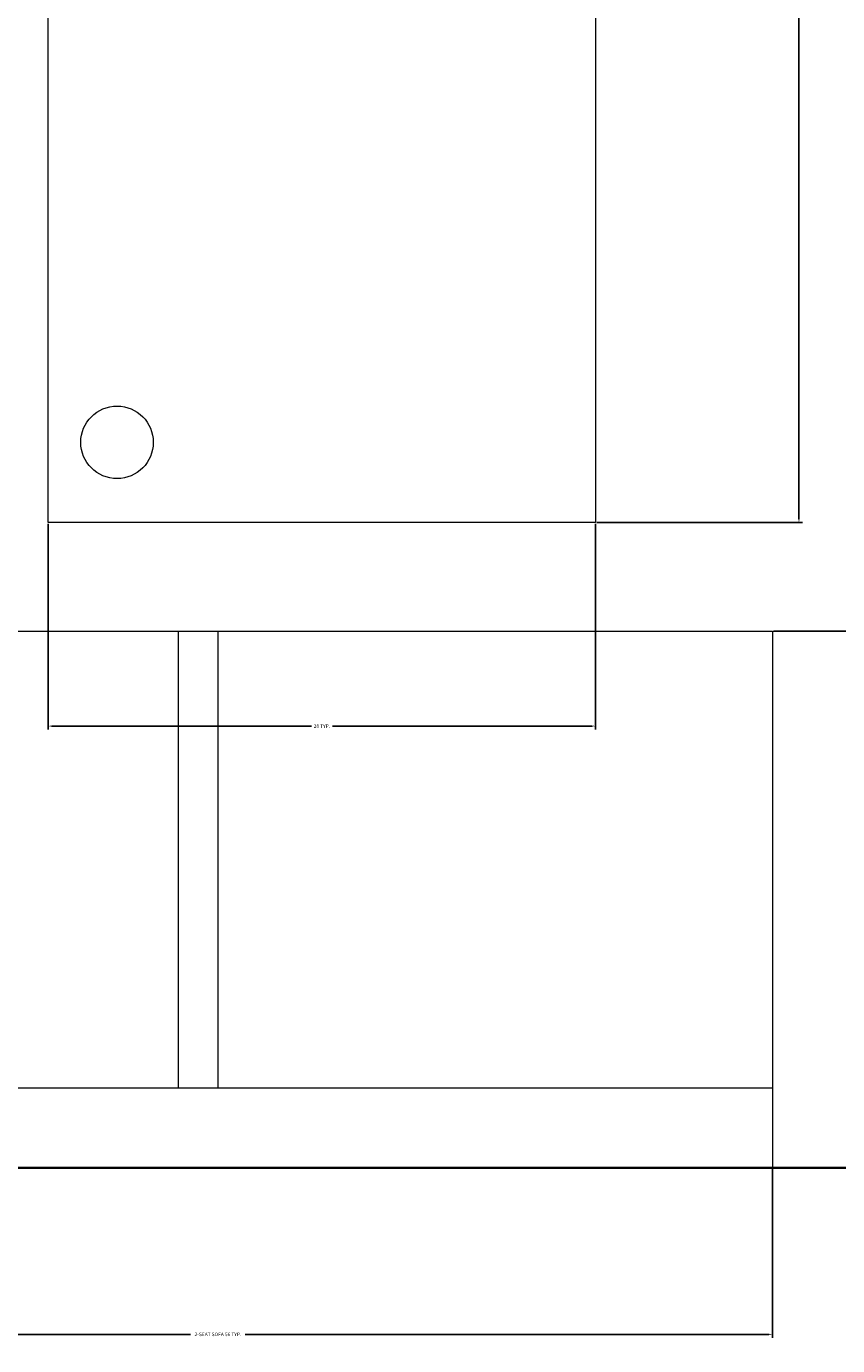
# Model space of a CAD drawing. Units: inches. Extents: x 108 to 613, y 1573 to 2319.
# Tile 5 of 11: x 365 to 406, y 1989 to 2055. Entities that reach past the tile are written whole.
import ezdxf

# ---------------------------------------------------------------- set-up
doc = ezdxf.new("R2010")
doc.units = ezdxf.units.IN
for name, color, linetype, lineweight in [('A-ANNO-DIMS', 2, 'Continuous', 18), ('furniture', 2, 'Continuous', 18), ('wall', 6, 'Continuous', 35)]:
    doc.layers.add(name, color=color, linetype=linetype, lineweight=lineweight)
doc.styles.get("Standard").update_dxf_attribs({"font": 'arial.ttf'})
doc.dimstyles.get("Standard").update_dxf_attribs({"dimtxt": 0.18, "dimasz": 0.18, "dimexe": 0.18, "dimexo": 0.0625, "dimgap": 0.09, "dimtad": 0, "dimtih": 1, "dimtoh": 1, "dimdec": 4, "dimzin": 0, "dimdsep": 46, "dimtxsty": 'Standard', "dimcen": 0.09, "dimadec": 0, "dimazin": 0, "dimtfac": 1, "dimtdec": 4, "dimtofl": 0, "dimtmove": 0, "dimatfit": 3, "dimfxl": 1, "dimtolj": 1, "dimtzin": 0, "dimarcsym": 0})

# ---------------------------------------------------------------- blocks, each defined once
blk = doc.blocks.new('COFFEE-TABLE')
blk.add_lwpolyline([(0, 68.458), (27.63, 68.458), (27.63, 0), (0, 0)], close=True)
blk.add_circle((3.474, 4.049), 1.83)
blk = doc.blocks.new('SOFA-2-SEAT')
for p, q in [((25.991, 27.084), (25.991, 4.025)), ((27.991, 27.084), (27.991, 4.025)), ((55.982, 4.025), (0, 4.025))]:
    blk.add_line(p, q)
blk.add_lwpolyline([(0, 27.084), (55.982, 27.084), (55.982, 0), (0, 0)], close=True)
blk = doc.blocks.new('*D29')
at = {"layer": 'A-ANNO-DIMS', "color": 0, "lineweight": -2, "transparency": 16777216}
for p, q in [((394.077, 2098.634), (404.464, 2098.634)), ((404.284, 2098.454), (404.284, 2064.588)), ((404.284, 2030.356), (404.284, 2064.222)), ((394.077, 2030.176), (404.464, 2030.176))]:
    blk.add_line(p, q, dxfattribs=at)
at = {"layer": 'A-ANNO-DIMS', "color": 0, "transparency": 16777216}
for points in [[(404.254, 2098.454), (404.314, 2098.454), (404.284, 2098.634)], [(404.254, 2030.356), (404.314, 2030.356), (404.284, 2030.176)]]:
    blk.add_solid(points, dxfattribs=at)
at = {"layer": 'Defpoints', "color": 0, "transparency": 16777216}
for p in [(394.015, 2098.634), (404.284, 2098.634), (394.015, 2030.176)]:
    blk.add_point(p, dxfattribs=at)
at = {"layer": 'A-ANNO-DIMS', "color": 0, "transparency": 16777216, "insert": (404.284, 2064.405), "char_height": 0.18, "attachment_point": 5}
blk.add_mtext('\\A1;COFFEE TABLE 68 TYP.', dxfattribs=at)
blk = doc.blocks.new('*D30')
at = {"layer": 'A-ANNO-DIMS', "color": 0, "lineweight": -2, "transparency": 16777216}
for p, q in [((366.385, 2030.114), (366.385, 2019.727)), ((394.015, 2030.114), (394.015, 2019.727)), ((366.565, 2019.907), (379.671, 2019.907)), ((393.835, 2019.907), (380.73, 2019.907))]:
    blk.add_line(p, q, dxfattribs=at)
at = {"layer": 'A-ANNO-DIMS', "color": 0, "transparency": 16777216}
for points in [[(366.565, 2019.937), (366.565, 2019.877), (366.385, 2019.907)], [(393.835, 2019.937), (393.835, 2019.877), (394.015, 2019.907)]]:
    blk.add_solid(points, dxfattribs=at)
at = {"layer": 'Defpoints', "color": 0, "transparency": 16777216}
for p in [(366.385, 2030.176), (394.015, 2030.176), (394.015, 2019.907)]:
    blk.add_point(p, dxfattribs=at)
at = {"layer": 'A-ANNO-DIMS', "color": 0, "transparency": 16777216, "insert": (380.2, 2019.907), "char_height": 0.18, "attachment_point": 5}
blk.add_mtext('\\A1;28 TYP.', dxfattribs=at)
blk = doc.blocks.new('*D33')
at = {"layer": 'A-ANNO-DIMS', "color": 0, "lineweight": -2, "transparency": 16777216}
for p, q in [((346.962, 1997.55), (346.962, 1989.035)), ((402.944, 1997.55), (402.944, 1989.035)), ((347.142, 1989.215), (373.571, 1989.215)), ((402.764, 1989.215), (376.335, 1989.215))]:
    blk.add_line(p, q, dxfattribs=at)
at = {"layer": 'A-ANNO-DIMS', "color": 0, "transparency": 16777216}
for points in [[(347.142, 1989.245), (347.142, 1989.185), (346.962, 1989.215)], [(402.764, 1989.245), (402.764, 1989.185), (402.944, 1989.215)]]:
    blk.add_solid(points, dxfattribs=at)
at = {"layer": 'Defpoints', "color": 0, "transparency": 16777216}
for p in [(346.962, 1997.612), (402.944, 1997.612), (402.944, 1989.215)]:
    blk.add_point(p, dxfattribs=at)
at = {"layer": 'A-ANNO-DIMS', "color": 0, "transparency": 16777216, "insert": (374.953, 1989.215), "char_height": 0.18, "attachment_point": 5}
blk.add_mtext('\\A1;2-SEAT SOFA 56 TYP.', dxfattribs=at)
blk = doc.blocks.new('*D34')
at = {"layer": 'A-ANNO-DIMS', "color": 0, "lineweight": -2, "transparency": 16777216}
for p, q in [((403.006, 2024.696), (411.521, 2024.696)), ((411.341, 2024.516), (411.341, 2011.335)), ((411.341, 1997.792), (411.341, 2010.974)), ((403.006, 1997.612), (411.521, 1997.612))]:
    blk.add_line(p, q, dxfattribs=at)
at = {"layer": 'A-ANNO-DIMS', "color": 0, "transparency": 16777216}
for points in [[(411.311, 2024.516), (411.371, 2024.516), (411.341, 2024.696)], [(411.311, 1997.792), (411.371, 1997.792), (411.341, 1997.612)]]:
    blk.add_solid(points, dxfattribs=at)
at = {"layer": 'Defpoints', "color": 0, "transparency": 16777216}
for p in [(402.944, 2024.696), (411.341, 2024.696), (402.944, 1997.612)]:
    blk.add_point(p, dxfattribs=at)
at = {"layer": 'A-ANNO-DIMS', "color": 0, "transparency": 16777216, "insert": (411.341, 2011.154), "char_height": 0.18, "attachment_point": 5}
blk.add_mtext('\\A1;27 TYP.', dxfattribs=at)

msp = doc.modelspace()

# ---------------------------------------------------------------- linework, layer by layer
at = {"layer": 'wall'}
msp.add_line((341.2753, 1997.6125), (431.2753, 1997.6125), dxfattribs=at)

# ---------------------------------------------------------------- block references
at = {"layer": 'furniture'}
for name, p in [('COFFEE-TABLE', (366.385, 2030.176)), ('SOFA-2-SEAT', (346.962, 1997.612))]:
    msp.add_blockref(name, p, dxfattribs=at)

# ---------------------------------------------------------------- dimensions: what is measured, and where the dimension line sits
at = {"layer": 'A-ANNO-DIMS'}
for base, p1, p2, text, picture, middle in [((404.2835, 2098.634), (394.0149, 2030.176), (394.0149, 2098.634), 'COFFEE TABLE <> TYP.', '*D29', (404.2835, 2064.405)), ((411.3411, 2024.6958), (402.9438, 1997.6125), (402.9438, 2024.6958), '<> TYP.', '*D34', (411.3411, 2011.1541))]:
    dim = msp.add_linear_dim(base=base, p1=p1, p2=p2, angle=90, text=text, dimstyle='Standard', override={"dimdec": 0, "dimlfac": 1, "dimrnd": 0, "dimzin": 0, "dimdsep": 46, "dimlunit": 2}, dxfattribs=at)
    dim.commit()
    dim.dimension.update_dxf_attribs({"geometry": picture, "text_midpoint": middle})
for base, p1, p2, text, picture, middle in [((394.0149, 2019.9074), (366.3854, 2030.176), (394.0149, 2030.176), '<> TYP.', '*D30', (380.2001, 2019.9074)), ((402.9438, 1989.2152), (346.9619, 1997.6125), (402.9438, 1997.6125), '2-SEAT SOFA <> TYP.', '*D33', (374.9528, 1989.2152))]:
    dim = msp.add_linear_dim(base=base, p1=p1, p2=p2, text=text, dimstyle='Standard', override={"dimdec": 0, "dimlfac": 1, "dimrnd": 0, "dimzin": 0, "dimdsep": 46, "dimlunit": 2}, dxfattribs=at)
    dim.commit()
    dim.dimension.update_dxf_attribs({"geometry": picture, "text_midpoint": middle})

doc.saveas('drawing.dxf')
